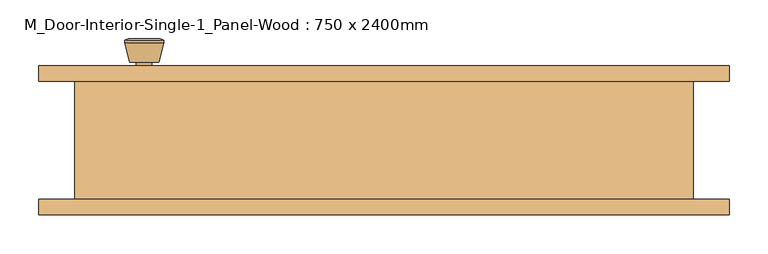
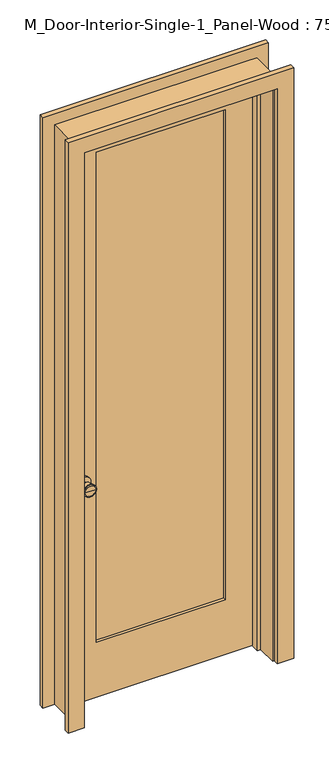
"""IFC4 building model written with IfcOpenShell, lengths in millimetres: door geometry, M_Door-Interior-Single-1_Panel-Wood : 750 x 2400mm."""

from ifc_helpers import new_model, si_unit, point, frame, frame_2d, origin, place, context, project, spatial, polyline, circle_curve, trimmed, segment, composite_curve, outline, extrude, faceted_brep, source, transform, mapped, element, save
from ifc_brep_helpers import plane_surface, cylinder_surface, revolved_surface, advanced_brep


def m_door_interior_single_1_panel_wood_750_x_2400mm_f8366a1a(model_context):
    return source(origin(), model_context, "Body", "SolidModel", [
        advanced_brep(
        [(-310.0, 32.025, 914.4), (-300.0, 32.025, 914.4), (-320.0, 32.025, 914.4), (-289.5241324, -16.975, 914.4), (-310.0, -16.975, 914.4), (-330.4758676, -16.975, 914.4), (-285.0, -15.1471319, 914.4), (-335.0, -15.1471319, 914.4), (-285.0, -11.6834537, 914.4), (-335.0, -11.6834537, 914.4), (-291.363764, 13.025, 914.4), (-328.636236, 13.025, 914.4), (-300.0, 13.025, 914.4), (-320.0, 13.025, 914.4)],
        [
            (0, 1),
            (1, 2, circle_curve(frame((-310.0, 32.025, 914.4), z_axis=(0.0, 1.0, 0.0), x_axis=(-1.0, 0.0, 0.0)), 10.0)),
            (2, 0),
            (2, 1, circle_curve(frame((-310.0, 32.025, 914.4), z_axis=(0.0, 1.0, 0.0), x_axis=(-1.0, 0.0, 0.0)), 10.0)),
            (3, 4),
            (4, 5),
            (5, 3, circle_curve(frame((-310.0, -16.975, 914.4), z_axis=(0.0, -1.0, 0.0), x_axis=(-1.0, 0.0, 0.0)), 20.4758676)),
            (3, 5, circle_curve(frame((-310.0, -16.975, 914.4), z_axis=(0.0, -1.0, 0.0), x_axis=(-1.0, 0.0, 0.0)), 20.4758676)),
            (6, 3),
            (5, 7),
            (7, 6, circle_curve(frame((-310.0, -15.1471319, 914.4), z_axis=(0.0, -1.0, 0.0), x_axis=(-1.0, 0.0, 0.0)), 25.0)),
            (6, 7, circle_curve(frame((-310.0, -15.1471319, 914.4), z_axis=(0.0, -1.0, 0.0), x_axis=(-1.0, 0.0, 0.0)), 25.0)),
            (8, 6),
            (7, 9),
            (9, 8, circle_curve(frame((-310.0, -11.6834537, 914.4), z_axis=(0.0, -1.0, 0.0), x_axis=(-1.0, 0.0, 0.0)), 25.0)),
            (8, 9, circle_curve(frame((-310.0, -11.6834537, 914.4), z_axis=(0.0, -1.0, 0.0), x_axis=(-1.0, 0.0, 0.0)), 25.0)),
            (10, 8),
            (9, 11),
            (11, 10, circle_curve(frame((-310.0, 13.025, 914.4), z_axis=(0.0, -1.0, 0.0), x_axis=(-1.0, 0.0, 0.0)), 18.636236)),
            (10, 11, circle_curve(frame((-310.0, 13.025, 914.4), z_axis=(0.0, -1.0, 0.0), x_axis=(-1.0, 0.0, 0.0)), 18.636236)),
            (12, 10),
            (11, 13),
            (13, 12, circle_curve(frame((-310.0, 13.025, 914.4), z_axis=(0.0, -1.0, 0.0), x_axis=(-1.0, 0.0, 0.0)), 10.0)),
            (12, 13, circle_curve(frame((-310.0, 13.025, 914.4), z_axis=(0.0, -1.0, 0.0), x_axis=(-1.0, 0.0, 0.0)), 10.0)),
            (1, 12),
            (13, 2),
        ],
        [
            plane_surface(frame((-310.0, 32.025, 914.4), z_axis=(0.0, 1.0, 0.0), x_axis=(-1.0, 0.0, 0.0))),
            plane_surface(frame((-310.0, -16.975, 914.4), z_axis=(0.0, -1.0, 0.0), x_axis=(-1.0, 0.0, 0.0))),
            revolved_surface(polyline([(-330.4758676, -16.975, 914.4), (-335.0, -15.1471319, 914.4)]), (-310.0, 32.025, 914.4), (0.0, 1.0, 0.0)),
            cylinder_surface(frame((-310.0, 32.025, 914.4), z_axis=(0.0, 1.0, 0.0), x_axis=(-1.0, 0.0, 0.0)), 25.0),
            revolved_surface(polyline([(-335.0, -11.6834537, 914.4), (-328.636236, 13.025, 914.4)]), (-310.0, 32.025, 914.4), (0.0, 1.0, 0.0)),
            plane_surface(frame((-310.0, 13.025, 914.4), z_axis=(0.0, 1.0, 0.0), x_axis=(-1.0, 0.0, 0.0))),
            cylinder_surface(frame((-310.0, 32.025, 914.4), z_axis=(0.0, 1.0, 0.0), x_axis=(-1.0, 0.0, 0.0)), 10.0),
        ],
        [
            (0, [[1, 2, 3]]),
            (0, [[-3, 4, -1]]),
            (1, [[5, 6, 7]]),
            (1, [[-6, -5, 8]]),
            (2, [[9, -7, 10, 11]]),
            (2, [[-10, -8, -9, 12]]),
            (3, [[13, -11, 14, 15]]),
            (3, [[-14, -12, -13, 16]]),
            (4, [[17, -15, 18, 19]]),
            (4, [[-18, -16, -17, 20]]),
            (5, [[21, -19, 22, 23]]),
            (5, [[-22, -20, -21, 24]]),
            (6, [[25, -23, 26, -2]]),
            (6, [[-26, -24, -25, -4]]),
        ],
    ),
        extrude(outline(composite_curve([segment(trimmed(circle_curve(frame_2d((914.4, -310.0)), 30.0), [point((914.4, -340.0))], [point((914.4, -280.0))], False, "CARTESIAN"), True, "CONTINUOUS"), segment(trimmed(circle_curve(frame_2d((914.4, -310.0)), 30.0), [point((914.4, -280.0))], [point((914.4, -340.0))], False, "CARTESIAN"), True, "CONTINUOUS")], self_intersect=False)), frame((0.0, 32.025, 0.0), z_axis=(0.0, 1.0, 0.0), x_axis=(0.0, 0.0, 1.0)), (0.0, 0.0, 1.0), 6.0),
        advanced_brep(
        [(-310.0, 79.025, 914.4), (-320.0, 79.025, 914.4), (-300.0, 79.025, 914.4), (-289.5241324, 128.025, 914.4), (-330.4758676, 128.025, 914.4), (-310.0, 128.025, 914.4), (-285.0, 126.1971319, 914.4), (-335.0, 126.1971319, 914.4), (-285.0, 122.7334537, 914.4), (-335.0, 122.7334537, 914.4), (-291.363764, 98.025, 914.4), (-328.636236, 98.025, 914.4), (-300.0, 98.025, 914.4), (-320.0, 98.025, 914.4)],
        [
            (0, 1),
            (1, 2, circle_curve(frame((-310.0, 79.025, 914.4), z_axis=(0.0, -1.0, 0.0), x_axis=(-1.0, 0.0, 0.0)), 10.0)),
            (2, 0),
            (2, 1, circle_curve(frame((-310.0, 79.025, 914.4), z_axis=(0.0, -1.0, 0.0), x_axis=(-1.0, 0.0, 0.0)), 10.0)),
            (3, 4, circle_curve(frame((-310.0, 128.025, 914.4), z_axis=(0.0, 1.0, 0.0), x_axis=(-1.0, 0.0, 0.0)), 20.4758676)),
            (4, 5),
            (5, 3),
            (4, 3, circle_curve(frame((-310.0, 128.025, 914.4), z_axis=(0.0, 1.0, 0.0), x_axis=(-1.0, 0.0, 0.0)), 20.4758676)),
            (6, 7, circle_curve(frame((-310.0, 126.1971319, 914.4), z_axis=(0.0, 1.0, 0.0), x_axis=(-1.0, 0.0, 0.0)), 25.0)),
            (7, 4),
            (3, 6),
            (7, 6, circle_curve(frame((-310.0, 126.1971319, 914.4), z_axis=(0.0, 1.0, 0.0), x_axis=(-1.0, 0.0, 0.0)), 25.0)),
            (8, 9, circle_curve(frame((-310.0, 122.7334537, 914.4), z_axis=(0.0, 1.0, 0.0), x_axis=(-1.0, 0.0, 0.0)), 25.0)),
            (9, 7),
            (6, 8),
            (9, 8, circle_curve(frame((-310.0, 122.7334537, 914.4), z_axis=(0.0, 1.0, 0.0), x_axis=(-1.0, 0.0, 0.0)), 25.0)),
            (10, 11, circle_curve(frame((-310.0, 98.025, 914.4), z_axis=(0.0, 1.0, 0.0), x_axis=(-1.0, 0.0, 0.0)), 18.636236)),
            (11, 9),
            (8, 10),
            (11, 10, circle_curve(frame((-310.0, 98.025, 914.4), z_axis=(0.0, 1.0, 0.0), x_axis=(-1.0, 0.0, 0.0)), 18.636236)),
            (12, 13, circle_curve(frame((-310.0, 98.025, 914.4), z_axis=(0.0, 1.0, 0.0), x_axis=(-1.0, 0.0, 0.0)), 10.0)),
            (13, 11),
            (10, 12),
            (13, 12, circle_curve(frame((-310.0, 98.025, 914.4), z_axis=(0.0, 1.0, 0.0), x_axis=(-1.0, 0.0, 0.0)), 10.0)),
            (1, 13),
            (12, 2),
        ],
        [
            plane_surface(frame((-310.0, 79.025, 914.4), z_axis=(0.0, -1.0, 0.0), x_axis=(-1.0, 0.0, 0.0))),
            plane_surface(frame((-310.0, 128.025, 914.4), z_axis=(0.0, 1.0, 0.0), x_axis=(-1.0, 0.0, 0.0))),
            revolved_surface(polyline([(-330.4758676, 128.025, 914.4), (-335.0, 126.1971319, 914.4)]), (-310.0, 79.025, 914.4), (0.0, -1.0, 0.0)),
            cylinder_surface(frame((-310.0, 79.025, 914.4), z_axis=(0.0, -1.0, 0.0), x_axis=(-1.0, 0.0, 0.0)), 25.0),
            revolved_surface(polyline([(-335.0, 122.7334537, 914.4), (-328.636236, 98.025, 914.4)]), (-310.0, 79.025, 914.4), (0.0, -1.0, 0.0)),
            plane_surface(frame((-310.0, 98.025, 914.4), z_axis=(0.0, -1.0, 0.0), x_axis=(-1.0, 0.0, 0.0))),
            cylinder_surface(frame((-310.0, 79.025, 914.4), z_axis=(0.0, -1.0, 0.0), x_axis=(-1.0, 0.0, 0.0)), 10.0),
        ],
        [
            (0, [[1, 2, 3]]),
            (0, [[-3, 4, -1]]),
            (1, [[5, 6, 7]]),
            (1, [[8, -7, -6]]),
            (2, [[9, 10, -5, 11]]),
            (2, [[12, -11, -8, -10]]),
            (3, [[13, 14, -9, 15]]),
            (3, [[16, -15, -12, -14]]),
            (4, [[17, 18, -13, 19]]),
            (4, [[20, -19, -16, -18]]),
            (5, [[21, 22, -17, 23]]),
            (5, [[24, -23, -20, -22]]),
            (6, [[-2, 25, -21, 26]]),
            (6, [[-4, -26, -24, -25]]),
        ],
    ),
        extrude(outline(composite_curve([segment(trimmed(circle_curve(frame_2d((914.4, -310.0)), 30.0), [point((914.4, -340.0))], [point((914.4, -280.0))], False, "CARTESIAN"), True, "CONTINUOUS"), segment(trimmed(circle_curve(frame_2d((914.4, -310.0)), 30.0), [point((914.4, -280.0))], [point((914.4, -340.0))], False, "CARTESIAN"), True, "CONTINUOUS")], self_intersect=False)), frame((0.0, 73.025, 0.0), z_axis=(0.0, 1.0, 0.0), x_axis=(0.0, 0.0, 1.0)), (0.0, 0.0, 1.0), 6.0),
        extrude(outline(polyline([(255.0, 49.6916667), (-255.0, 49.6916667), (-255.0, 61.3583333), (255.0, 61.3583333), (255.0, 49.6916667)])), frame((0.0, 0.0, 230.0), z_axis=(0.0, 0.0, 1.0), x_axis=(1.0, 0.0, 0.0)), (0.0, 0.0, 1.0), 2050.0),
        extrude(outline(polyline([(2400.0, -375.0), (0.0, -375.0), (0.0, 375.0), (2400.0, 375.0), (2400.0, -375.0)]), holes=[polyline([(2280.0, -255.0), (2280.0, 255.0), (230.0, 255.0), (230.0, -255.0), (2280.0, -255.0)])]), frame((0.0, 38.025, 0.0), z_axis=(0.0, 1.0, 0.0), x_axis=(0.0, 0.0, 1.0)), (0.0, 0.0, 1.0), 35.0),
        faceted_brep([(400.0, 73.025, 0.0), (400.0, -79.375, 0.0), (375.0, -79.375, 0.0), (375.0, 3.1, 0.0), (362.3, 3.1, 0.0), (362.3, 38.025, 0.0), (375.0, 38.025, 0.0), (375.0, 73.025, 0.0), (400.0, 73.025, 2425.0), (400.0, -79.375, 2425.0), (-400.0, -79.375, 2425.0), (-400.0, -79.375, 0.0), (-375.0, -79.375, 0.0), (-375.0, -79.375, 2400.0), (375.0, -79.375, 2400.0), (375.0, 3.1, 2400.0), (-375.0, 3.1, 2400.0), (-375.0, 3.1, 0.0), (-362.3, 3.1, 0.0), (-362.3, 3.1, 2387.3), (362.3, 3.1, 2387.3), (362.3, 38.025, 2387.3), (-362.3, 38.025, 2387.3), (-362.3, 38.025, 0.0), (-375.0, 38.025, 0.0), (-375.0, 38.025, 2400.0), (375.0, 38.025, 2400.0), (375.0, 73.025, 2400.0), (-375.0, 73.025, 2400.0), (-375.0, 73.025, 0.0), (-400.0, 73.025, 0.0), (-400.0, 73.025, 2425.0)], [[[0, 1, 2, 3, 4, 5, 6, 7]], [[1, 0, 8, 9]], [[2, 1, 9, 10, 11, 12, 13, 14]], [[3, 2, 14, 15]], [[4, 3, 15, 16, 17, 18, 19, 20]], [[5, 4, 20, 21]], [[6, 5, 21, 22, 23, 24, 25, 26]], [[7, 6, 26, 27]], [[0, 7, 27, 28, 29, 30, 31, 8]], [[9, 8, 31, 10]], [[15, 14, 13, 16]], [[21, 20, 19, 22]], [[27, 26, 25, 28]], [[30, 29, 24, 23, 18, 17, 12, 11]], [[10, 31, 30, 11]], [[16, 13, 12, 17]], [[22, 19, 18, 23]], [[28, 25, 24, 29]]]),
        extrude(outline(polyline([(0.0, 381.35), (0.0, 446.35), (2471.35, 446.35), (2471.35, -446.35), (0.0, -446.35), (0.0, -381.35), (2406.35, -381.35), (2406.35, 381.35), (0.0, 381.35)])), frame((0.0, -99.375, 0.0), z_axis=(0.0, 1.0, 0.0), x_axis=(0.0, 0.0, 1.0)), (0.0, 0.0, 1.0), 20.0),
        extrude(outline(polyline([(0.0, 381.35), (0.0, 446.35), (2471.35, 446.35), (2471.35, -446.35), (0.0, -446.35), (0.0, -381.35), (2406.35, -381.35), (2406.35, 381.35), (0.0, 381.35)])), frame((0.0, 73.025, 0.0), z_axis=(0.0, 1.0, 0.0), x_axis=(0.0, 0.0, 1.0)), (0.0, 0.0, 1.0), 20.0),
    ])


if __name__ == "__main__":
    model = new_model("IFC4")
    model_context = context("Model", 3, world=origin())
    ifc_project = project(units=[si_unit("LENGTHUNIT", "METRE", prefix="MILLI")], contexts=[model_context])
    site = spatial("IfcSite", under=ifc_project)
    building = spatial("IfcBuilding", under=site)
    placement = place(None, origin())
    m_door_interior_single_1_panel_wood_750_x_2400mm_shape = m_door_interior_single_1_panel_wood_750_x_2400mm_f8366a1a(model_context)
    element("IfcDoor", 1, ObjectType="M_Door-Interior-Single-1_Panel-Wood : 750 x 2400mm", at=placement, inside=building, context=model_context, shape_type="MappedRepresentation", body=[
        mapped(m_door_interior_single_1_panel_wood_750_x_2400mm_shape, transform((0.0, 0.0, 0.0), x_axis=(1.0, 0.0, 0.0), y_axis=(0.0, 1.0, 0.0), z_axis=(0.0, 0.0, 1.0))),
    ])
    save(model, "model.ifc")

# Revit data of these elements
# Type "M_Door-Interior-Single-1_Panel-Wood : 750 x 2400mm"
#   Type Mark = "8"
#   Assembly Code = "C1020300"
#   Analytic Construction = "Wooden"
#   Top Rail = 0' - 4.72441"
#   Thickness = 0' - 1.37795"
#   Thermal Resistance (R) = 2.5876 (h·ft²·°F)/BTU
#   Swing Angle [instance default] = 90.00°
#   Stiles = 0' - 4.72441"
#   Rough Width = 2' - 7.49606"
#   Rough Height = 7' - 11.47244"
#   Height = 7' - 10.48819"
#   Width = 2' - 5.52756"
#   Heat Transfer Coefficient (U) = 0.3865 BTU/(h·ft²·°F)
#   Bottom Rail = 0' - 9.05512"
#   Trim Material = Cherry
#   Panel Material = Cherry
#   Frame Material = Cherry
#   Door Handle Material = Aluminum
#   Visual Light Transmittance = 0
#   Solar Heat Gain Coefficient = 0
#   Wall Closure = (empty or 0)
#   Function = (empty or 0)
# Element 1 (IfcDoor, "M_Door-Interior-Single-1_Panel-Wood : 750 x 2400mm")
#   Materials on its faces: "Cherry", "Aluminum"
# Materials
#   "Cherry": class "Wood", colour RGB 226 177 128, transparency 0, Description = "Prunus Serotina", Cost = 0
#   "Aluminum": class "Metal", colour RGB 247 247 247, transparency 0, Description = "Aluminum 6061", Cost = 0
